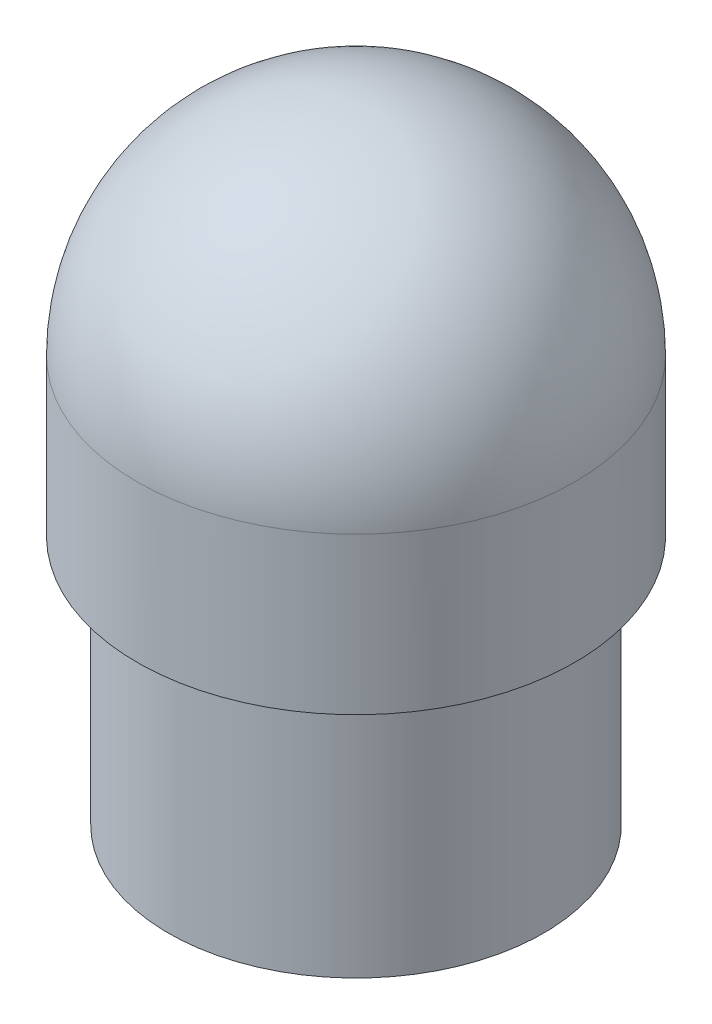
ISO-10303-21;
HEADER;
FILE_DESCRIPTION(('STEP AP214'),'2;1');
FILE_NAME('part.step','',(''),(''),'','','');
FILE_SCHEMA(('AUTOMOTIVE_DESIGN { 1 0 10303 214 1 1 1 1 }'));
ENDSEC;
DATA;
#1=APPLICATION_CONTEXT('core data for automotive mechanical design processes');
#2=APPLICATION_PROTOCOL_DEFINITION('international standard','automotive_design',2000,#1);
#3=PRODUCT_CONTEXT('',#1,'mechanical');
#4=PRODUCT('Part','Part','',(#3));
#5=PRODUCT_RELATED_PRODUCT_CATEGORY('part','',(#4));
#6=PRODUCT_DEFINITION_FORMATION('','',#4);
#7=PRODUCT_DEFINITION_CONTEXT('part definition',#1,'design');
#8=PRODUCT_DEFINITION('design','',#6,#7);
#9=PRODUCT_DEFINITION_SHAPE('','',#8);
#10=(LENGTH_UNIT() NAMED_UNIT(*) SI_UNIT(.MILLI.,.METRE.));
#11=(NAMED_UNIT(*) PLANE_ANGLE_UNIT() SI_UNIT($,.RADIAN.));
#12=(NAMED_UNIT(*) SI_UNIT($,.STERADIAN.) SOLID_ANGLE_UNIT());
#13=UNCERTAINTY_MEASURE_WITH_UNIT(LENGTH_MEASURE(1.E-05),#10,'distance_accuracy_value','');
#14=(GEOMETRIC_REPRESENTATION_CONTEXT(3) GLOBAL_UNCERTAINTY_ASSIGNED_CONTEXT((#13)) GLOBAL_UNIT_ASSIGNED_CONTEXT((#10,
#11,#12)) REPRESENTATION_CONTEXT('',''));
#15=CARTESIAN_POINT('',(0.,0.,0.));
#16=DIRECTION('',(0.,0.,1.));
#17=DIRECTION('',(1.,0.,0.));
#18=AXIS2_PLACEMENT_3D('',#15,#16,#17);
#19=CARTESIAN_POINT('',(0.,0.,0.));
#20=DIRECTION('',(0.,1.,0.));
#21=DIRECTION('',(-1.,0.,0.));
#22=AXIS2_PLACEMENT_3D('',#19,#20,#21);
#23=PLANE('',#22);
#24=CARTESIAN_POINT('',(0.,0.,0.));
#25=DIRECTION('',(0.,1.,0.));
#26=DIRECTION('',(-1.,0.,0.));
#27=AXIS2_PLACEMENT_3D('',#24,#25,#26);
#28=CIRCLE('',#27,15.);
#29=CARTESIAN_POINT('',(-15.,0.,0.));
#30=VERTEX_POINT('',#29);
#31=EDGE_CURVE('E10',#30,#30,#28,.T.);
#32=ORIENTED_EDGE('',*,*,#31,.F.);
#33=EDGE_LOOP('',(#32));
#34=FACE_BOUND('',#33,.T.);
#35=ADVANCED_FACE('F40',(#34),#23,.F.);
#36=CARTESIAN_POINT('',(0.,50.,0.));
#37=DIRECTION('',(0.,1.,0.));
#38=DIRECTION('',(-1.,0.,0.));
#39=AXIS2_PLACEMENT_3D('',#36,#37,#38);
#40=CYLINDRICAL_SURFACE('',#39,15.);
#41=CARTESIAN_POINT('',(0.,20.,0.));
#42=DIRECTION('',(0.,1.,0.));
#43=DIRECTION('',(-1.,0.,0.));
#44=AXIS2_PLACEMENT_3D('',#41,#42,#43);
#45=CIRCLE('',#44,15.);
#46=CARTESIAN_POINT('',(-15.,20.,0.));
#47=VERTEX_POINT('',#46);
#48=EDGE_CURVE('E43',#47,#47,#45,.T.);
#49=ORIENTED_EDGE('',*,*,#48,.F.);
#50=EDGE_LOOP('',(#49));
#51=FACE_BOUND('',#50,.T.);
#52=ORIENTED_EDGE('',*,*,#31,.T.);
#53=EDGE_LOOP('',(#52));
#54=FACE_BOUND('',#53,.T.);
#55=ADVANCED_FACE('F70',(#51,#54),#40,.T.);
#56=CARTESIAN_POINT('',(15.,20.,0.));
#57=DIRECTION('',(0.,1.,0.));
#58=DIRECTION('',(-1.,0.,0.));
#59=AXIS2_PLACEMENT_3D('',#56,#57,#58);
#60=PLANE('',#59);
#61=CARTESIAN_POINT('',(0.,20.,0.));
#62=DIRECTION('',(0.,1.,0.));
#63=DIRECTION('',(-1.,0.,0.));
#64=AXIS2_PLACEMENT_3D('',#61,#62,#63);
#65=CIRCLE('',#64,17.5);
#66=CARTESIAN_POINT('',(-17.5,20.,0.));
#67=VERTEX_POINT('',#66);
#68=EDGE_CURVE('E50',#67,#67,#65,.T.);
#69=ORIENTED_EDGE('',*,*,#68,.F.);
#70=EDGE_LOOP('',(#69));
#71=FACE_BOUND('',#70,.T.);
#72=ORIENTED_EDGE('',*,*,#48,.T.);
#73=EDGE_LOOP('',(#72));
#74=FACE_BOUND('',#73,.T.);
#75=ADVANCED_FACE('F65',(#71,#74),#60,.F.);
#76=CARTESIAN_POINT('',(0.,50.,0.));
#77=DIRECTION('',(0.,1.,0.));
#78=DIRECTION('',(-1.,0.,0.));
#79=AXIS2_PLACEMENT_3D('',#76,#77,#78);
#80=CYLINDRICAL_SURFACE('',#79,17.5);
#81=CARTESIAN_POINT('',(0.,32.5,0.));
#82=DIRECTION('',(0.,1.,0.));
#83=DIRECTION('',(-1.,0.,0.));
#84=AXIS2_PLACEMENT_3D('',#81,#82,#83);
#85=CIRCLE('',#84,17.5);
#86=CARTESIAN_POINT('',(-17.5,32.5,0.));
#87=VERTEX_POINT('',#86);
#88=EDGE_CURVE('E51',#87,#87,#85,.T.);
#89=ORIENTED_EDGE('',*,*,#88,.F.);
#90=EDGE_LOOP('',(#89));
#91=FACE_BOUND('',#90,.T.);
#92=ORIENTED_EDGE('',*,*,#68,.T.);
#93=EDGE_LOOP('',(#92));
#94=FACE_BOUND('',#93,.T.);
#95=ADVANCED_FACE('F56',(#91,#94),#80,.T.);
#96=CARTESIAN_POINT('',(0.,32.5,0.));
#97=DIRECTION('',(0.,1.,0.));
#98=DIRECTION('',(1.,0.,0.));
#99=AXIS2_PLACEMENT_3D('',#96,#97,#98);
#100=SPHERICAL_SURFACE('',#99,17.5);
#101=ORIENTED_EDGE('',*,*,#88,.T.);
#102=EDGE_LOOP('',(#101));
#103=FACE_BOUND('',#102,.T.);
#104=ADVANCED_FACE('F60',(#103),#100,.T.);
#105=CLOSED_SHELL('',(#35,#55,#75,#95,#104));
#106=MANIFOLD_SOLID_BREP('B2',#105);
#107=ADVANCED_BREP_SHAPE_REPRESENTATION('',(#18,#106),#14);
#108=SHAPE_DEFINITION_REPRESENTATION(#9,#107);
ENDSEC;
END-ISO-10303-21;
